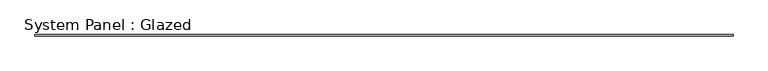
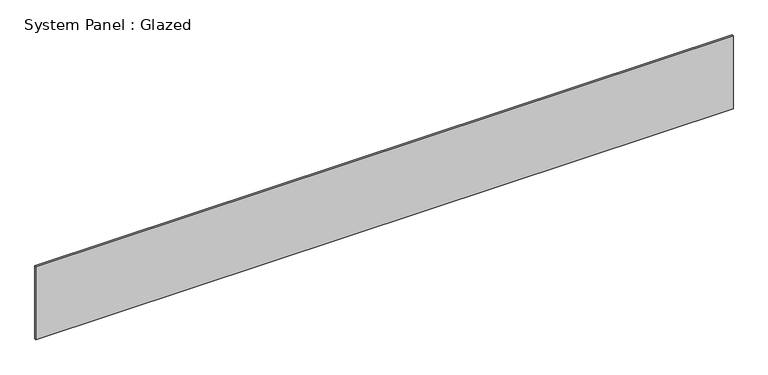
"""IFC4 building model written with IfcOpenShell, lengths in millimetres: plate geometry, System Panel : Glazed."""

from ifc_helpers import new_model, si_unit, origin, origin_with_axes, place, context, project, spatial, polyline, outline, extrude, source, transform, mapped, element, save


def system_panel_glazed_281b5f8b(model_context):
    return source(origin(), model_context, "Body", "SweptSolid", [
        extrude(outline(polyline([(6884.5614633, 19.05), (-6884.5614633, 19.05), (-6884.5614633, 44.45), (6884.5614633, 44.45), (6884.5614633, 19.05)])), origin_with_axes(), (0.0, 0.0, 1.0), 1524.0),
    ])


if __name__ == "__main__":
    model = new_model("IFC4")
    model_context = context("Model", 3, world=origin())
    ifc_project = project(units=[si_unit("LENGTHUNIT", "METRE", prefix="MILLI")], contexts=[model_context])
    site = spatial("IfcSite", under=ifc_project)
    building = spatial("IfcBuilding", under=site)
    placement = place(None, origin())
    system_panel_glazed_shape = system_panel_glazed_281b5f8b(model_context)
    element("IfcPlate", 1, ObjectType="System Panel : Glazed", at=placement, inside=building, context=model_context, shape_type="MappedRepresentation", body=[
        mapped(system_panel_glazed_shape, transform((0.0, 0.0, 0.0), x_axis=(1.0, 0.0, 0.0), y_axis=(0.0, 1.0, 0.0), z_axis=(0.0, 0.0, 1.0))),
    ])
    save(model, "model.ifc")

# Revit data of these elements
# Type "System Panel : Glazed"
#   Construction Type Id = "GSP4R"
#   Analytic Construction = "1/8 in Pilkington single glazing"
#   Visual Light Transmittance = 0.9
#   Solar Heat Gain Coefficient = 0.86
#   Heat Transfer Coefficient (U) = 1.18115 BTU/(h·ft²·°F)
# Element 1 (IfcPlate, "System Panel : Glazed")
#   Materials on its faces: "Glass"
# Materials
#   "Glass": class "Glass", colour RGB 0 128 192, transparency 0.75, Description = "Soda Lime Glass", Cost = 0
